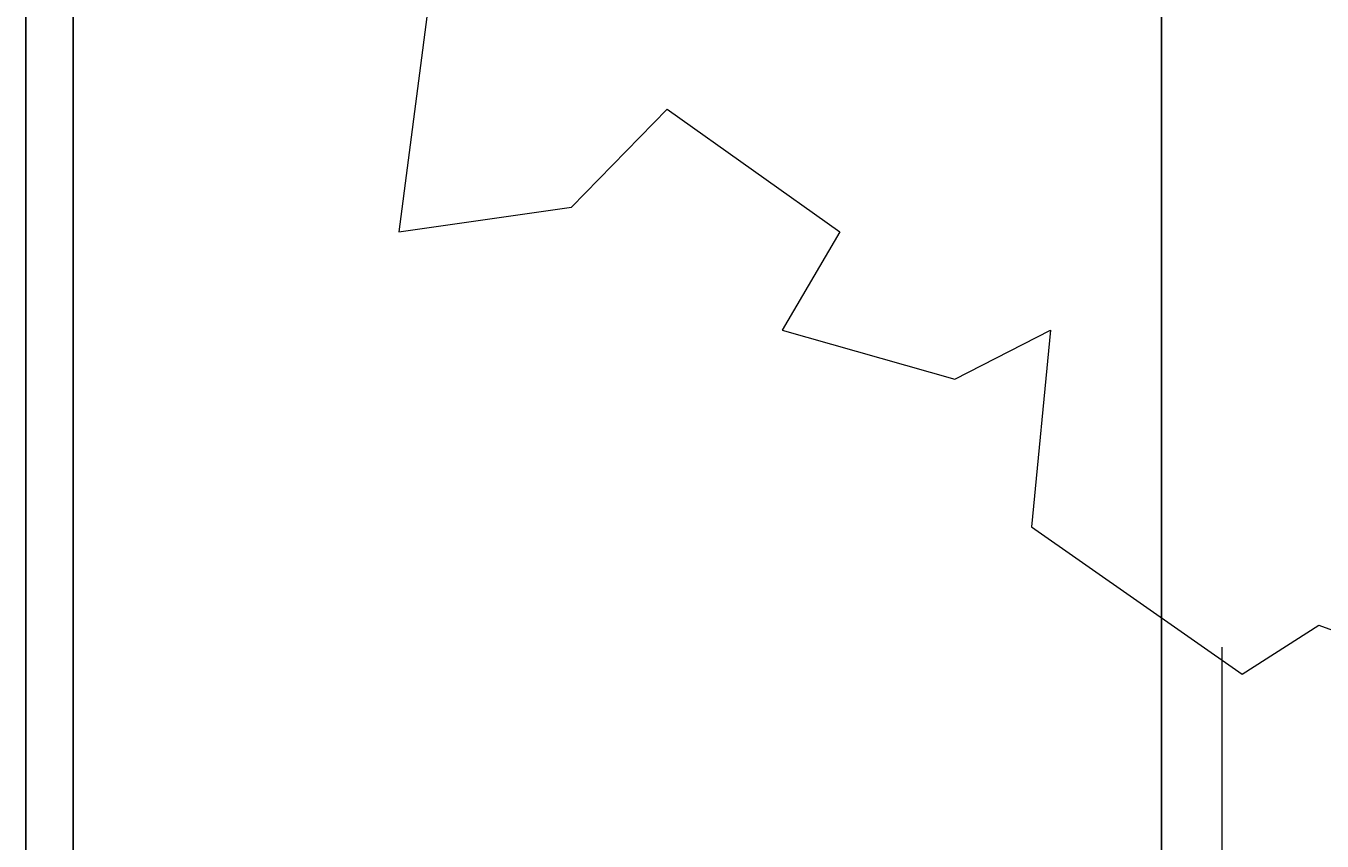
# Model space of a CAD drawing. Units: inches. Extents: x -26 to 776, y -22 to 650.
# Tile 42 of 62: x 426 to 506, y 52 to 102. Entities that reach past the tile are written whole.
import ezdxf

# ---------------------------------------------------------------- set-up
doc = ezdxf.new("R2010")
doc.units = ezdxf.units.IN
doc.header["$MEASUREMENT"] = 0
doc.layers.add('A-ANNO-DIMS', color=2, linetype='Continuous', lineweight=18)
doc.layers.add('L-PLNT-TREE', color=94, linetype='Continuous', lineweight=18)
doc.styles.get("Standard").update_dxf_attribs({"font": 'arial.ttf'})
doc.dimstyles.get("Standard").update_dxf_attribs({"dimtxt": 0.5625, "dimasz": 0.18, "dimexe": 0.18, "dimexo": 0.0625, "dimgap": 0.09, "dimtad": 0, "dimtih": 1, "dimtoh": 1, "dimdec": 4, "dimzin": 0, "dimdsep": 46, "dimlunit": 4, "dimtxsty": 'Standard', "dimcen": 0.09, "dimadec": 0, "dimazin": 0, "dimtfac": 1, "dimtdec": 4, "dimtofl": 0, "dimtmove": 0, "dimatfit": 3, "dimfxl": 1, "dimtolj": 1, "dimtzin": 0, "dimarcsym": 0})

# ---------------------------------------------------------------- blocks, each defined once
blk = doc.blocks.new('Tree - type 2 deciduous elevation')
for points in [[(-30.36, 44.975), (-31.51, 36.128), (-26.334, 36.865), (-23.459, 39.814), (-18.283, 36.128), (-20.008, 33.178), (-14.832, 31.704), (-11.956, 33.178), (-12.531, 27.28), (-6.205, 22.856), (-3.905, 24.331), (0.121, 22.856), (8.173, 26.543), (11.624, 25.068), (12.199, 27.28), (21.4, 34.653), (19.675, 39.077), (23.701, 44.975)], [(-6.813, 23.669), (-6.813, 11.669), (-8.627, 0)]]:
    blk.add_lwpolyline(points)
blk = doc.blocks.new('*D20')
at = {"layer": 'A-ANNO-DIMS', "color": 0, "lineweight": -2, "transparency": 16777216}
for p, q in [((425.806, 455.472), (775.335, 455.472)), ((775.155, 455.292), (775.155, 235.854)), ((775.155, 15.662), (775.155, 235.1)), ((425.806, 15.482), (775.335, 15.482))]:
    blk.add_line(p, q, dxfattribs=at)
at = {"layer": 'A-ANNO-DIMS', "color": 0, "transparency": 16777216}
for points in [[(775.125, 455.292), (775.185, 455.292), (775.155, 455.472)], [(775.125, 15.662), (775.185, 15.662), (775.155, 15.482)]]:
    blk.add_solid(points, dxfattribs=at)
at = {"layer": 'Defpoints', "color": 0, "transparency": 16777216}
for p in [(425.743, 455.472), (775.155, 455.472), (425.743, 15.482)]:
    blk.add_point(p, dxfattribs=at)
at = {"layer": 'A-ANNO-DIMS', "color": 0, "transparency": 16777216, "insert": (775.155, 235.477), "char_height": 0.5625, "attachment_point": 5}
blk.add_mtext('\\A1;440', dxfattribs=at)
blk = doc.blocks.new('*D30')
at = {"layer": 'A-ANNO-DIMS', "color": 0, "lineweight": -2, "transparency": 16777216}
for p, q in [((280.68, 144.836), (775.335, 144.836)), ((775.155, 144.656), (775.155, 86.007)), ((775.155, 26.604), (775.155, 85.253)), ((280.68, 26.424), (775.335, 26.424))]:
    blk.add_line(p, q, dxfattribs=at)
at = {"layer": 'A-ANNO-DIMS', "color": 0, "transparency": 16777216}
for points in [[(775.125, 144.656), (775.185, 144.656), (775.155, 144.836)], [(775.125, 26.604), (775.185, 26.604), (775.155, 26.424)]]:
    blk.add_solid(points, dxfattribs=at)
at = {"layer": 'Defpoints', "color": 0, "transparency": 16777216}
for p in [(280.617, 144.836), (775.155, 144.836), (280.617, 26.424)]:
    blk.add_point(p, dxfattribs=at)
at = {"layer": 'A-ANNO-DIMS', "color": 0, "transparency": 16777216, "insert": (775.155, 85.63), "char_height": 0.5625, "attachment_point": 5}
blk.add_mtext('\\A1;118.41', dxfattribs=at)
blk = doc.blocks.new('*D39')
at = {"layer": 'A-ANNO-DIMS', "color": 0, "lineweight": -2, "transparency": 16777216}
for p, q in [((289.242, 15.545), (289.242, 649.856)), ((289.422, 649.676), (356.478, 649.676)), ((425.563, 649.676), (358.508, 649.676)), ((425.743, 15.545), (425.743, 649.856))]:
    blk.add_line(p, q, dxfattribs=at)
at = {"layer": 'A-ANNO-DIMS', "color": 0, "transparency": 16777216}
for points in [[(289.422, 649.706), (289.422, 649.646), (289.242, 649.676)], [(425.563, 649.706), (425.563, 649.646), (425.743, 649.676)]]:
    blk.add_solid(points, dxfattribs=at)
at = {"layer": 'Defpoints', "color": 0, "transparency": 16777216}
for p in [(425.743, 649.676), (289.242, 15.482), (425.743, 15.482)]:
    blk.add_point(p, dxfattribs=at)
at = {"layer": 'A-ANNO-DIMS', "color": 0, "transparency": 16777216, "insert": (357.493, 649.676), "char_height": 0.5625, "attachment_point": 5}
blk.add_mtext('\\A1;136.5', dxfattribs=at)
blk = doc.blocks.new('*D40')
at = {"layer": 'A-ANNO-DIMS', "color": 0, "lineweight": -2, "transparency": 16777216}
for p, q in [((425.743, 15.545), (425.743, 649.856)), ((425.923, 649.676), (459.646, 649.676)), ((495.451, 649.676), (461.728, 649.676)), ((495.631, 15.545), (495.631, 649.856))]:
    blk.add_line(p, q, dxfattribs=at)
at = {"layer": 'A-ANNO-DIMS', "color": 0, "transparency": 16777216}
for points in [[(425.923, 649.706), (425.923, 649.646), (425.743, 649.676)], [(495.451, 649.706), (495.451, 649.646), (495.631, 649.676)]]:
    blk.add_solid(points, dxfattribs=at)
at = {"layer": 'Defpoints', "color": 0, "transparency": 16777216}
for p in [(495.631, 649.676), (425.743, 15.482), (495.631, 15.482)]:
    blk.add_point(p, dxfattribs=at)
at = {"layer": 'A-ANNO-DIMS', "color": 0, "transparency": 16777216, "insert": (460.687, 649.676), "char_height": 0.5625, "attachment_point": 5}
blk.add_mtext('\\A1;69.89', dxfattribs=at)
blk = doc.blocks.new('*D47')
at = {"layer": 'A-ANNO-DIMS', "color": 0, "lineweight": -2, "transparency": 16777216}
for p, q in [((584.343, 199.901), (584.343, -21.315)), ((428.648, 180.243), (428.648, -21.315)), ((428.828, -21.135), (505.483, -21.135)), ((584.163, -21.135), (507.508, -21.135))]:
    blk.add_line(p, q, dxfattribs=at)
at = {"layer": 'A-ANNO-DIMS', "color": 0, "transparency": 16777216}
for points in [[(428.828, -21.105), (428.828, -21.165), (428.648, -21.135)], [(584.163, -21.105), (584.163, -21.165), (584.343, -21.135)]]:
    blk.add_solid(points, dxfattribs=at)
at = {"layer": 'Defpoints', "color": 0, "transparency": 16777216}
for p in [(584.343, 199.963), (428.648, 180.305), (584.343, -21.135)]:
    blk.add_point(p, dxfattribs=at)
at = {"layer": 'A-ANNO-DIMS', "color": 0, "transparency": 16777216, "insert": (506.496, -21.135), "char_height": 0.5625, "attachment_point": 5}
blk.add_mtext('\\A1;155.7', dxfattribs=at)

msp = doc.modelspace()

# ---------------------------------------------------------------- block references
at = {"layer": 'L-PLNT-TREE', "xscale": 2.050905272406618, "yscale": 2.050905272406618, "zscale": 2.050905272406618}
msp.add_blockref('Tree - type 2 deciduous elevation', (513.3241, 15.4824), dxfattribs=at)

# ---------------------------------------------------------------- dimensions: what is measured, and where the dimension line sits
at = {"layer": 'A-ANNO-DIMS'}
for base, p1, p2, override, picture, middle in [((425.7434, 649.6763), (289.2424, 15.4824), (425.7434, 15.4824), {"dimdec": 1, "dimlfac": 1, "dimrnd": 0, "dimzin": 0, "dimdsep": 46, "dimlunit": 2}, '*D39', (357.4929, 649.6763)), ((495.6309, 649.6763), (425.7434, 15.4824), (495.6309, 15.4824), {"dimdec": 2, "dimlfac": 1, "dimrnd": 0, "dimzin": 0, "dimdsep": 46, "dimlunit": 2}, '*D40', (460.6872, 649.6763)), ((584.3428, -21.1349), (428.6484, 180.3054), (584.3428, 199.9634), {"dimdec": 1, "dimlfac": 1, "dimrnd": 0, "dimzin": 0, "dimdsep": 46, "dimlunit": 2}, '*D47', (506.4956, -21.1349))]:
    dim = msp.add_linear_dim(base=base, p1=p1, p2=p2, dimstyle='Standard', override=override, dxfattribs=at)
    dim.commit()
    dim.dimension.update_dxf_attribs({"geometry": picture, "text_midpoint": middle})
for base, p1, p2, override, picture, middle in [((775.1553, 455.4717), (425.7434, 15.4824), (425.7434, 455.4717), {"dimdec": 0, "dimlfac": 1, "dimrnd": 0, "dimzin": 0, "dimdsep": 46, "dimlunit": 2}, '*D20', (775.1553, 235.477)), ((775.1553, 144.8359), (280.6173, 26.4239), (280.6173, 144.8359), {"dimdec": 2, "dimlfac": 1, "dimrnd": 0, "dimzin": 0, "dimdsep": 46, "dimlunit": 2}, '*D30', (775.1553, 85.6299))]:
    dim = msp.add_linear_dim(base=base, p1=p1, p2=p2, angle=90, dimstyle='Standard', override=override, dxfattribs=at)
    dim.commit()
    dim.dimension.update_dxf_attribs({"geometry": picture, "text_midpoint": middle})

doc.saveas('drawing.dxf')
